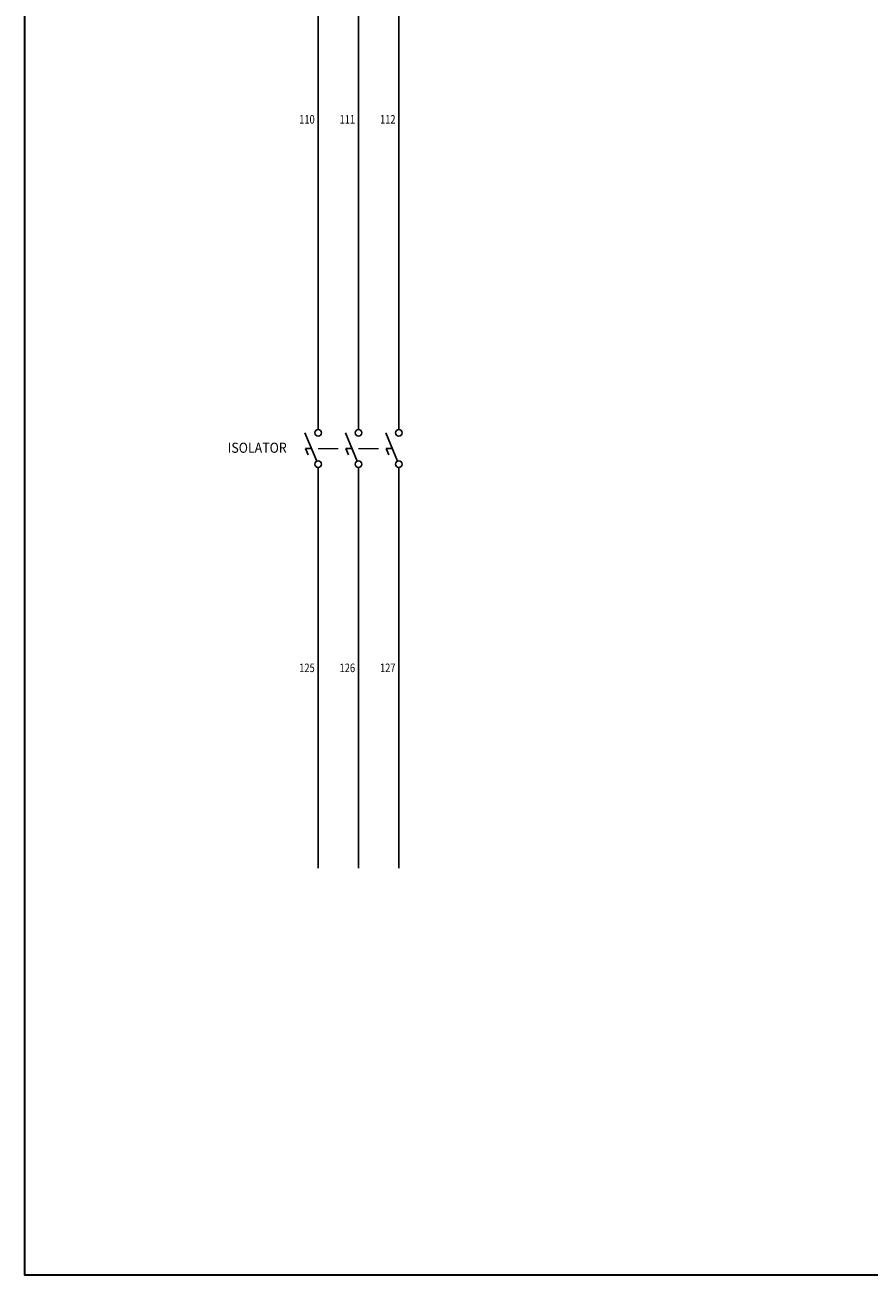
# Model space of a CAD drawing. Units: inches. Extents: x 12.5 to 62, y 4.7 to 37.4.
# Tile 1 of 5: x 12.5 to 24.9, y 4.7 to 23.1. Entities that reach past the tile are written whole.
import ezdxf
from ezdxf.enums import TextEntityAlignment as Align

# ---------------------------------------------------------------- set-up
doc = ezdxf.new("R2010")
doc.units = ezdxf.units.IN
doc.header["$MEASUREMENT"] = 0
for name, color, linetype, lineweight in [('16AWG-BLU', 182, 'Continuous', 25), ('16AWG-GRNYEL', 60, 'Continuous', 25), ('16AWG-RED', 1, 'Continuous', 25), ('E-ANNO-TTLB', 7, 'Continuous', 35), ('LINK', 9, 'Continuous', 13), ('SYMS', 7, 'Continuous', 25), ('WIRENO', 72, 'Continuous', 18)]:
    doc.layers.add(name, color=color, linetype=linetype, lineweight=lineweight)
doc.layers.add('TAGS', color=150, linetype='Continuous')
doc.styles.add('WD', font='romans.shx')

# ---------------------------------------------------------------- blocks, each defined once
blk = doc.blocks.new('VDS11')
for p, q in [((-0.016, -0.157), (-0.163, 0.195)), ((-0.081, 0), (-0.156, 0)), ((-0.124, -0.078), (-0.156, 0))]:
    blk.add_line(p, q)
for centre in [(0, 0.194), (0, -0.194)]:
    blk.add_circle(centre, 0.0403)
at = {"style": 'WD'}
for tag, height, flags, p in [('TERM01', 0.125, 8, (-0.069, 0.258)), ('CONTACT', 0.0125, 9, (-0.083, -0.067)), ('FAMILY', 0.0125, 9, (-0.1, -0.046)), ('MFG', 0.0125, 9, (-0.1, -0.11)), ('CAT', 0.0125, 9, (-0.1, -0.091))]:
    blk.add_attdef(tag, text='', height=height, dxfattribs=dict(at, flags=flags)).set_placement(p, align=Align.RIGHT)
for tag, width, p in [('INST', 0.7, (-0.391, 0.312)), ('LOC', 0.7, (-0.391, 0.125)), ('TAG1', 0.9, (-0.388, -0.054)), ('RATING1', 0.7, (-0.388, -0.234)), ('DESC1', 0.7, (-0.387, -0.422)), ('DESC2', 0.7, (-0.388, -0.609))]:
    blk.add_attdef(tag, text='', height=0.125, dxfattribs=dict(at, width=width)).set_placement(p, align=Align.RIGHT)
at = {"style": 'WD', "flags": 1}
for tag, p in [('X2TERM01', (0, 0.234)), ('X8TERM02', (0, -0.234))]:
    blk.add_attdef(tag, p, '', height=0.0125, dxfattribs=at)
at = {"style": 'WD'}
for tag, p in [('X4LINK', (-0.254, 0)), ('X1LINK', (0, 0))]:
    blk.add_attdef(tag, p, '', height=0.0125, dxfattribs=at)
at = {"style": 'WD', "width": 0.7}
blk.add_attdef('XREF', (0.161, -0.047), '', height=0.125, dxfattribs=at)
at = {"style": 'WD', "flags": 9}
blk.add_attdef('ASSYCODE', text='', height=0.0125, dxfattribs=at).set_placement((-0.115, -0.137), align=Align.CENTER)
at = {"style": 'WD', "flags": 8}
blk.add_attdef('TERM02', text='', height=0.125, dxfattribs=at).set_placement((-0.051, -0.267), align=Align.TOP_RIGHT)
blk = doc.blocks.new('WD_WNV')
at = {"style": 'WD', "width": 0.8}
blk.add_attdef('WIRENO', text='', height=0.125, dxfattribs=at).set_placement((-0.05, 0), align=Align.MIDDLE_RIGHT)
at = {"style": 'WD', "flags": 1}
for tag, p in [('W01USER', (-0.062, 0.094)), ('W02USER', (-0.062, 0.086)), ('W03USER', (-0.062, 0.078)), ('W04USER', (-0.062, 0.07)), ('W05USER', (-0.062, 0.062)), ('W06USER', (-0.062, 0.055)), ('W07USER', (-0.062, 0.047)), ('W08USER', (-0.062, 0.039)), ('W09USER', (-0.062, 0.031)), ('W10USER', (-0.062, 0.023))]:
    blk.add_attdef(tag, text='', height=0.005, dxfattribs=at).set_placement(p, align=Align.CENTER)

msp = doc.modelspace()

# ---------------------------------------------------------------- linework, layer by layer
at = {"layer": '16AWG-BLU'}
for p, q in [((18.014, 26.274), (18.014, 17.161)), ((18.014, 16.605), (18.014, 10.716))]:
    msp.add_line(p, q, dxfattribs=at)
at = {"layer": '16AWG-GRNYEL'}
for p, q in [((17.421, 26.274), (17.421, 17.161)), ((17.421, 16.605), (17.421, 10.716))]:
    msp.add_line(p, q, dxfattribs=at)
at = {"layer": '16AWG-RED'}
for p, q in [((16.828, 26.274), (16.828, 17.161)), ((16.828, 16.605), (16.828, 10.716))]:
    msp.add_line(p, q, dxfattribs=at)
at = {"layer": 'E-ANNO-TTLB'}
msp.add_lwpolyline([(12.524, 37.377), (62.033, 37.377), (62.033, 4.741), (12.524, 4.741)], close=True, dxfattribs=at)
at = {"layer": 'LINK'}
for points in [[(16.828, 16.883), (17.12, 16.883)], [(17.421, 16.883), (17.713, 16.883)]]:
    msp.add_lwpolyline(points, dxfattribs=at)

# ---------------------------------------------------------------- block references
at = {"layer": 'SYMS'}
ref = msp.add_blockref('VDS11', (16.828, 16.883), dxfattribs=dict(at, xscale=1.186465831832244, yscale=1.186465831832244, zscale=1.186465831832244))
ref.add_attrib('TAG1', 'ISOLATOR', dxfattribs={"layer": 'TAGS', "height": 0.1483, "style": 'WD', "width": 0.9}).set_placement((16.367, 16.819), align=Align.RIGHT)
at = {"layer": 'SYMS', "xscale": 1.186465831832244, "yscale": 1.186465831832244, "zscale": 1.186465831832244}
for p in [(17.421, 16.883), (18.014, 16.883)]:
    msp.add_blockref('VDS11', p, dxfattribs=at)
at = {"layer": 'WIRENO'}
ref = msp.add_blockref('WD_WNV', (16.828, 21.717), dxfattribs=at)
ref.add_attrib('WIRENO', '110', dxfattribs={"linetype": 'Continuous', "height": 0.125, "style": 'WD', "width": 0.8}).set_placement((16.778, 21.717), align=Align.MIDDLE_RIGHT)
ref = msp.add_blockref('WD_WNV', (17.421, 21.717), dxfattribs=at)
ref.add_attrib('WIRENO', '111', dxfattribs={"linetype": 'Continuous', "height": 0.125, "style": 'WD', "width": 0.8}).set_placement((17.371, 21.717), align=Align.MIDDLE_RIGHT)
ref = msp.add_blockref('WD_WNV', (18.014, 21.717), dxfattribs=at)
ref.add_attrib('WIRENO', '112', dxfattribs={"linetype": 'Continuous', "height": 0.125, "style": 'WD', "width": 0.8}).set_placement((17.964, 21.717), align=Align.MIDDLE_RIGHT)
ref = msp.add_blockref('WD_WNV', (16.828, 13.66), dxfattribs=at)
ref.add_attrib('WIRENO', '125', dxfattribs={"linetype": 'Continuous', "height": 0.125, "style": 'WD', "width": 0.8}).set_placement((16.778, 13.66), align=Align.MIDDLE_RIGHT)
ref = msp.add_blockref('WD_WNV', (17.421, 13.66), dxfattribs=at)
ref.add_attrib('WIRENO', '126', dxfattribs={"linetype": 'Continuous', "height": 0.125, "style": 'WD', "width": 0.8}).set_placement((17.371, 13.66), align=Align.MIDDLE_RIGHT)
ref = msp.add_blockref('WD_WNV', (18.014, 13.66), dxfattribs=at)
ref.add_attrib('WIRENO', '127', dxfattribs={"linetype": 'Continuous', "height": 0.125, "style": 'WD', "width": 0.8}).set_placement((17.964, 13.66), align=Align.MIDDLE_RIGHT)

doc.saveas('drawing.dxf')
